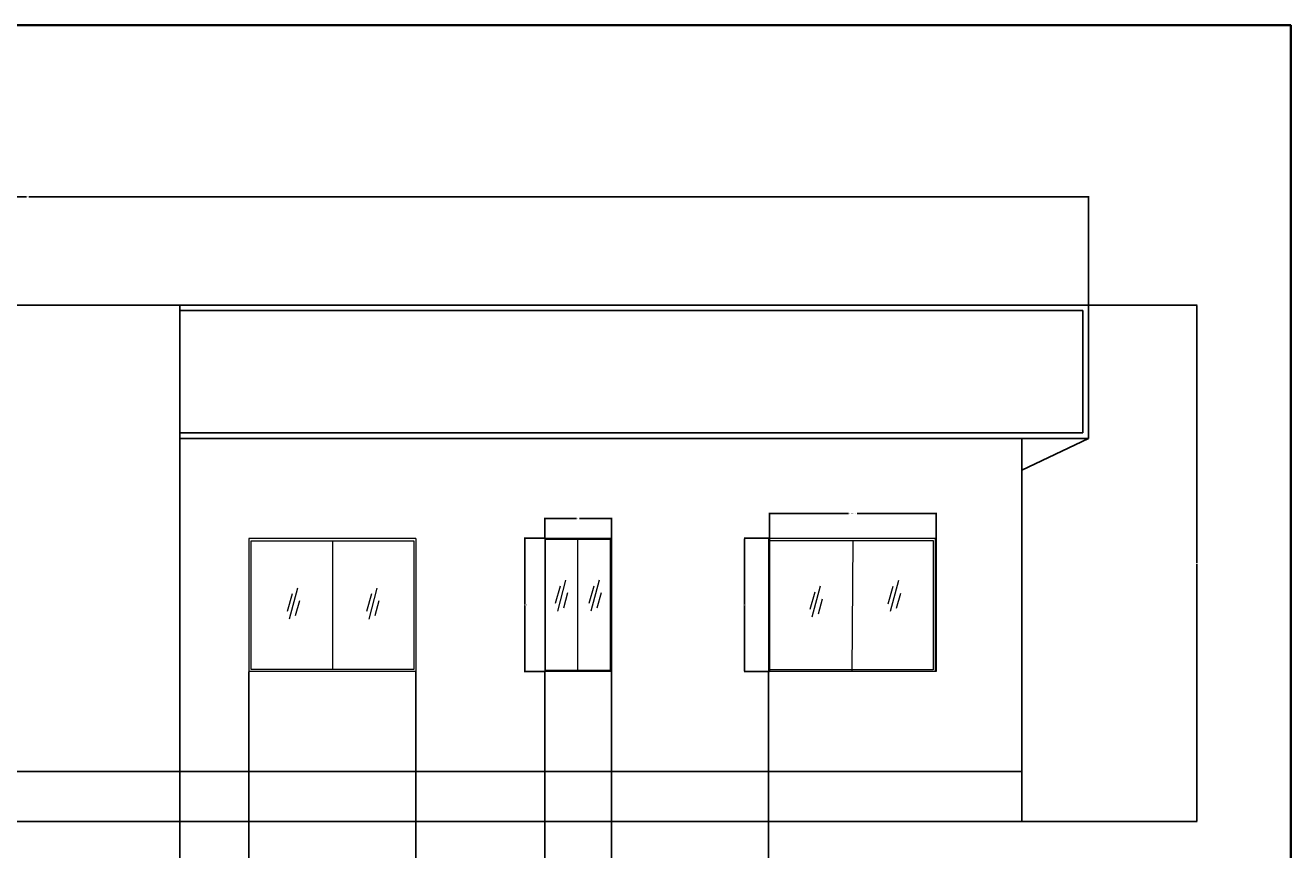
# Model space of a CAD drawing. Units: inches. Extents: x 2314 to 3223, y 1382 to 2735.
# Tile 14 of 14: x 2767 to 3223, y 2439 to 2735. Entities that reach past the tile are written whole.
import ezdxf

# ---------------------------------------------------------------- set-up
doc = ezdxf.new("R2010")
doc.units = ezdxf.units.IN
for name, color, linetype, lineweight in [('A-ANNO-DIMS', 2, 'Continuous', 18), ('A-ANNO-TTLB', 7, 'Continuous', 35), ('A-ELEV', 7, 'Continuous', 25), ('A-GLAZ-ELEV', 4, 'Continuous', 18)]:
    doc.layers.add(name, color=color, linetype=linetype, lineweight=lineweight)
doc.styles.get("Standard").update_dxf_attribs({"font": 'arial.ttf'})
doc.dimstyles.get("Standard").update_dxf_attribs({"dimtxt": 0.18, "dimasz": 0.18, "dimexe": 0.18, "dimexo": 0.0625, "dimgap": 0.09, "dimtad": 0, "dimtih": 1, "dimtoh": 1, "dimdec": 4, "dimzin": 0, "dimdsep": 46, "dimtxsty": 'Standard', "dimcen": 0.09, "dimadec": 0, "dimazin": 0, "dimtfac": 1, "dimtdec": 4, "dimtofl": 0, "dimtmove": 0, "dimatfit": 3, "dimfxl": 1, "dimtolj": 1, "dimtzin": 0, "dimarcsym": 0})

# ---------------------------------------------------------------- blocks, each defined once
blk = doc.blocks.new('WIN-ELEV-60X48-DIVIDED')
for p, q in [((0, 48), (0, 0)), ((60, 48), (0, 48)), ((30.07, 47.13), (30.07, 0.71)), ((60, 48), (60, 0)), ((60, 0), (0, 0))]:
    blk.add_line(p, q)
blk.add_lwpolyline([(0.83, 47.13), (59.31, 47.13), (59.31, 0.71), (0.83, 0.71)], close=True)
blk = doc.blocks.new('WIN-ELEV-60X48-FRAME-SASH')
for p, q in [((0, 48), (0, 0)), ((60, 48), (0, 48)), ((60, 48), (60, 0)), ((60, 0), (0, 0))]:
    blk.add_line(p, q)
blk.add_lwpolyline([(0.54, 47.23), (59.34, 47.23), (59.34, 0.63), (0.54, 0.63)], close=True)
blk = doc.blocks.new('WIN-ELEV-24X48-FRAME')
for p, q in [((0, 48), (0, 0)), ((24, 48), (0, 48)), ((24, 48), (24, 0)), ((24, 0), (0, 0))]:
    blk.add_line(p, q)
blk = doc.blocks.new('WIN-ELEV-60X48-FRAME')
for p, q in [((0, 48), (0, 0)), ((60, 48), (0, 48)), ((60, 48), (60, 0)), ((60, 0), (0, 0))]:
    blk.add_line(p, q)
blk = doc.blocks.new('GLASS-REFLECTION-MARK')
for p, q in [((3.77, 11.17), (0.81, 0)), ((1.83, 9.04), (0, 2.74)), ((4.5, 6.57), (2.99, 1.12))]:
    blk.add_line(p, q)
blk = doc.blocks.new('*D25')
at = {"layer": 'A-ANNO-DIMS', "color": 0, "lineweight": -2, "transparency": 16777216}
for p, q in [((2954.16, 2550.68), (2946.84, 2550.68)), ((2947.02, 2550.5), (2947.02, 2526.86)), ((2947.02, 2502.86), (2947.02, 2526.5)), ((2954.16, 2502.68), (2946.84, 2502.68))]:
    blk.add_line(p, q, dxfattribs=at)
at = {"layer": 'A-ANNO-DIMS', "color": 0, "transparency": 16777216}
for points in [[(2946.99, 2550.5), (2947.05, 2550.5), (2947.02, 2550.68)], [(2946.99, 2502.86), (2947.05, 2502.86), (2947.02, 2502.68)]]:
    blk.add_solid(points, dxfattribs=at)
at = {"layer": 'Defpoints', "color": 0, "transparency": 16777216}
for p in [(2947.02, 2550.68), (2954.22, 2550.68), (2954.22, 2502.68)]:
    blk.add_point(p, dxfattribs=at)
at = {"layer": 'A-ANNO-DIMS', "color": 0, "transparency": 16777216, "insert": (2947.02, 2526.68), "char_height": 0.18, "attachment_point": 5}
blk.add_mtext('\\A1;WINDOW 48 TYP.', dxfattribs=at)
blk = doc.blocks.new('*D26')
at = {"layer": 'A-ANNO-DIMS', "color": 0, "lineweight": -2, "transparency": 16777216}
for p, q in [((2954.22, 2550.74), (2954.22, 2558.06)), ((2954.4, 2557.88), (2965.69, 2557.88)), ((2978.04, 2557.88), (2966.75, 2557.88)), ((2978.22, 2550.74), (2978.22, 2558.06))]:
    blk.add_line(p, q, dxfattribs=at)
at = {"layer": 'A-ANNO-DIMS', "color": 0, "transparency": 16777216}
for points in [[(2954.4, 2557.91), (2954.4, 2557.85), (2954.22, 2557.88)], [(2978.04, 2557.91), (2978.04, 2557.85), (2978.22, 2557.88)]]:
    blk.add_solid(points, dxfattribs=at)
at = {"layer": 'Defpoints', "color": 0, "transparency": 16777216}
for p in [(2978.22, 2557.88), (2954.22, 2550.68), (2978.22, 2550.68)]:
    blk.add_point(p, dxfattribs=at)
at = {"layer": 'A-ANNO-DIMS', "color": 0, "transparency": 16777216, "insert": (2966.22, 2557.88), "char_height": 0.18, "attachment_point": 5}
blk.add_mtext('\\A1;24 TYP.', dxfattribs=at)
blk = doc.blocks.new('*D27')
at = {"layer": 'A-ANNO-DIMS', "color": 0, "lineweight": -2, "transparency": 16777216}
for p, q in [((3035.12, 2550.74), (3035.12, 2559.86)), ((3035.3, 2559.68), (3063.52, 2559.68)), ((3094.94, 2559.68), (3066.71, 2559.68)), ((3095.12, 2550.74), (3095.12, 2559.86))]:
    blk.add_line(p, q, dxfattribs=at)
at = {"layer": 'A-ANNO-DIMS', "color": 0, "transparency": 16777216}
for points in [[(3035.3, 2559.71), (3035.3, 2559.65), (3035.12, 2559.68)], [(3094.94, 2559.71), (3094.94, 2559.65), (3095.12, 2559.68)]]:
    blk.add_solid(points, dxfattribs=at)
at = {"layer": 'Defpoints', "color": 0, "transparency": 16777216}
for p in [(3095.12, 2559.68), (3035.12, 2550.68), (3095.12, 2550.68)]:
    blk.add_point(p, dxfattribs=at)
at = {"layer": 'A-ANNO-DIMS', "color": 0, "transparency": 16777216, "insert": (3065.12, 2559.68), "char_height": 0.18, "attachment_point": 5}
blk.add_mtext('\\A1;WINDOW FRAME 60 TYP.', dxfattribs=at)
blk = doc.blocks.new('*D28')
at = {"layer": 'A-ANNO-DIMS', "color": 0, "lineweight": -2, "transparency": 16777216}
for p, q in [((3035.05, 2550.68), (3025.94, 2550.68)), ((3026.12, 2550.5), (3026.12, 2526.86)), ((3026.12, 2502.86), (3026.12, 2526.5)), ((3035.05, 2502.68), (3025.94, 2502.68))]:
    blk.add_line(p, q, dxfattribs=at)
at = {"layer": 'A-ANNO-DIMS', "color": 0, "transparency": 16777216}
for points in [[(3026.09, 2550.5), (3026.15, 2550.5), (3026.12, 2550.68)], [(3026.09, 2502.86), (3026.15, 2502.86), (3026.12, 2502.68)]]:
    blk.add_solid(points, dxfattribs=at)
at = {"layer": 'Defpoints', "color": 0, "transparency": 16777216}
for p in [(3026.12, 2550.68), (3035.12, 2550.68), (3035.12, 2502.68)]:
    blk.add_point(p, dxfattribs=at)
at = {"layer": 'A-ANNO-DIMS', "color": 0, "transparency": 16777216, "insert": (3026.12, 2526.68), "char_height": 0.18, "attachment_point": 5}
blk.add_mtext('\\A1;48 TYP.', dxfattribs=at)
blk = doc.blocks.new('*D46')
at = {"layer": 'A-ANNO-DIMS', "color": 0, "lineweight": -2, "transparency": 16777216}
for p, q in [((2386.39, 2634.74), (2386.39, 2673.86)), ((2386.57, 2673.68), (2767.75, 2673.68)), ((3149.71, 2673.68), (2768.54, 2673.68)), ((3149.89, 2634.74), (3149.89, 2673.86))]:
    blk.add_line(p, q, dxfattribs=at)
at = {"layer": 'A-ANNO-DIMS', "color": 0, "transparency": 16777216}
for points in [[(2386.57, 2673.71), (2386.57, 2673.65), (2386.39, 2673.68)], [(3149.71, 2673.71), (3149.71, 2673.65), (3149.89, 2673.68)]]:
    blk.add_solid(points, dxfattribs=at)
at = {"layer": 'Defpoints', "color": 0, "transparency": 16777216}
for p in [(3149.89, 2673.68), (2386.39, 2634.68), (3149.89, 2634.68)]:
    blk.add_point(p, dxfattribs=at)
at = {"layer": 'A-ANNO-DIMS', "color": 0, "transparency": 16777216, "insert": (2768.14, 2673.68), "char_height": 0.18, "attachment_point": 5}
blk.add_mtext('\\A1;763.5', dxfattribs=at)
blk = doc.blocks.new('*D47')
at = {"layer": 'A-ANNO-DIMS', "color": 0, "lineweight": -2, "transparency": 16777216}
for p, q in [((3149.96, 2634.68), (3189.07, 2634.68)), ((3188.89, 2634.5), (3188.89, 2541.86)), ((3188.89, 2448.86), (3188.89, 2541.5)), ((3125.96, 2448.68), (3189.07, 2448.68))]:
    blk.add_line(p, q, dxfattribs=at)
at = {"layer": 'A-ANNO-DIMS', "color": 0, "transparency": 16777216}
for points in [[(3188.86, 2634.5), (3188.92, 2634.5), (3188.89, 2634.68)], [(3188.86, 2448.86), (3188.92, 2448.86), (3188.89, 2448.68)]]:
    blk.add_solid(points, dxfattribs=at)
at = {"layer": 'Defpoints', "color": 0, "transparency": 16777216}
for p in [(3149.89, 2634.68), (3125.89, 2448.68), (3188.89, 2448.68)]:
    blk.add_point(p, dxfattribs=at)
at = {"layer": 'A-ANNO-DIMS', "color": 0, "transparency": 16777216, "insert": (3188.89, 2541.68), "char_height": 0.18, "attachment_point": 5}
blk.add_mtext('\\A1;186', dxfattribs=at)
blk = doc.blocks.new('*D56')
at = {"layer": 'A-ANNO-DIMS', "color": 0, "lineweight": -2, "transparency": 16777216}
for p, q in [((2717.89, 2466.62), (2717.89, 2371.63)), ((2822.89, 2466.62), (2822.89, 2371.63)), ((2718.07, 2371.81), (2770.11, 2371.81)), ((2822.71, 2371.81), (2770.67, 2371.81))]:
    blk.add_line(p, q, dxfattribs=at)
at = {"layer": 'A-ANNO-DIMS', "color": 0, "transparency": 16777216}
for points in [[(2718.07, 2371.84), (2718.07, 2371.78), (2717.89, 2371.81)], [(2822.71, 2371.84), (2822.71, 2371.78), (2822.89, 2371.81)]]:
    blk.add_solid(points, dxfattribs=at)
at = {"layer": 'Defpoints', "color": 0, "transparency": 16777216}
for p in [(2717.89, 2466.68), (2822.89, 2466.68), (2822.89, 2371.81)]:
    blk.add_point(p, dxfattribs=at)
at = {"layer": 'A-ANNO-DIMS', "color": 0, "transparency": 16777216, "insert": (2770.39, 2371.81), "char_height": 0.18, "attachment_point": 5}
blk.add_mtext('\\A1;105', dxfattribs=at)
blk = doc.blocks.new('*D57')
at = {"layer": 'A-ANNO-DIMS', "color": 0, "lineweight": -2, "transparency": 16777216}
for p, q in [((2847.78, 2502.62), (2847.78, 2371.63)), ((2822.89, 2466.62), (2822.89, 2371.63)), ((2823.07, 2371.81), (2834.94, 2371.81)), ((2847.6, 2371.81), (2835.73, 2371.81))]:
    blk.add_line(p, q, dxfattribs=at)
at = {"layer": 'A-ANNO-DIMS', "color": 0, "transparency": 16777216}
for points in [[(2823.07, 2371.84), (2823.07, 2371.78), (2822.89, 2371.81)], [(2847.6, 2371.84), (2847.6, 2371.78), (2847.78, 2371.81)]]:
    blk.add_solid(points, dxfattribs=at)
at = {"layer": 'Defpoints', "color": 0, "transparency": 16777216}
for p in [(2847.78, 2502.68), (2822.89, 2466.68), (2847.78, 2371.81)]:
    blk.add_point(p, dxfattribs=at)
at = {"layer": 'A-ANNO-DIMS', "color": 0, "transparency": 16777216, "insert": (2835.34, 2371.81), "char_height": 0.18, "attachment_point": 5}
blk.add_mtext('\\A1;24.89', dxfattribs=at)
blk = doc.blocks.new('*D58')
at = {"layer": 'A-ANNO-DIMS', "color": 0, "lineweight": -2, "transparency": 16777216}
for p, q in [((2907.78, 2502.62), (2907.78, 2371.63)), ((2954.22, 2502.62), (2954.22, 2371.63)), ((2907.96, 2371.81), (2930.61, 2371.81)), ((2954.04, 2371.81), (2931.4, 2371.81))]:
    blk.add_line(p, q, dxfattribs=at)
at = {"layer": 'A-ANNO-DIMS', "color": 0, "transparency": 16777216}
for points in [[(2907.96, 2371.84), (2907.96, 2371.78), (2907.78, 2371.81)], [(2954.04, 2371.84), (2954.04, 2371.78), (2954.22, 2371.81)]]:
    blk.add_solid(points, dxfattribs=at)
at = {"layer": 'Defpoints', "color": 0, "transparency": 16777216}
for p in [(2907.78, 2502.68), (2954.22, 2502.68), (2954.22, 2371.81)]:
    blk.add_point(p, dxfattribs=at)
at = {"layer": 'A-ANNO-DIMS', "color": 0, "transparency": 16777216, "insert": (2931, 2371.81), "char_height": 0.18, "attachment_point": 5}
blk.add_mtext('\\A1;46.44', dxfattribs=at)
blk = doc.blocks.new('*D59')
at = {"layer": 'A-ANNO-DIMS', "color": 0, "lineweight": -2, "transparency": 16777216}
for p, q in [((2978.22, 2502.62), (2978.22, 2371.63)), ((3034.7, 2502.62), (3034.7, 2371.63)), ((2978.4, 2371.81), (3006.07, 2371.81)), ((3034.52, 2371.81), (3006.85, 2371.81))]:
    blk.add_line(p, q, dxfattribs=at)
at = {"layer": 'A-ANNO-DIMS', "color": 0, "transparency": 16777216}
for points in [[(2978.4, 2371.84), (2978.4, 2371.78), (2978.22, 2371.81)], [(3034.52, 2371.84), (3034.52, 2371.78), (3034.7, 2371.81)]]:
    blk.add_solid(points, dxfattribs=at)
at = {"layer": 'Defpoints', "color": 0, "transparency": 16777216}
for p in [(2978.22, 2502.68), (3034.7, 2502.68), (3034.7, 2371.81)]:
    blk.add_point(p, dxfattribs=at)
at = {"layer": 'A-ANNO-DIMS', "color": 0, "transparency": 16777216, "insert": (3006.46, 2371.81), "char_height": 0.18, "attachment_point": 5}
blk.add_mtext('\\A1;56.47', dxfattribs=at)

msp = doc.modelspace()

# ---------------------------------------------------------------- linework, layer by layer
at = {"layer": 'A-ANNO-TTLB'}
msp.add_lwpolyline([(2314.008, 2735.417), (3222.6676, 2735.417), (3222.6676, 1382.0876), (2314.008, 1382.0876)], close=True, dxfattribs=at)
at = {"layer": 'A-ELEV'}
for p, q in [((3149.8927, 2634.6793), (2386.3927, 2634.6793)), ((2822.8927, 2586.6793), (2822.8927, 2634.6793)), ((2822.8927, 2632.6793), (3147.8927, 2632.6793)), ((3147.8927, 2632.6793), (3147.8927, 2588.6793)), ((3149.8927, 2586.6793), (3149.8927, 2634.6793)), ((3147.8927, 2588.6793), (2822.8927, 2588.6793)), ((2822.8927, 2586.6793), (2822.8927, 2466.6793)), ((3149.8927, 2586.6793), (2822.8927, 2586.6793)), ((3125.8927, 2586.6793), (3125.8927, 2448.6793)), ((3149.8927, 2586.6793), (3125.8927, 2575.1733)), ((3125.8927, 2466.6793), (2410.3927, 2466.6793)), ((3125.8927, 2448.6793), (2410.3927, 2448.6793))]:
    msp.add_line(p, q, dxfattribs=at)
at = {"layer": 'A-GLAZ-ELEV'}
for p, q in [((2966.1716, 2503.0629), (2966.1716, 2550.3487)), ((3065.116, 2549.9127), (3064.6958, 2502.6793))]:
    msp.add_line(p, q, dxfattribs=at)
msp.add_lwpolyline([(2954.547, 2550.3487), (2977.7963, 2550.3487), (2977.7963, 2503.0629), (2954.547, 2503.0629)], close=True, dxfattribs=at)

# ---------------------------------------------------------------- block references
for name, p in [('WIN-ELEV-60X48-DIVIDED', (2847.783, 2502.6793)), ('WIN-ELEV-60X48-FRAME', (2847.783, 2502.6793)), ('WIN-ELEV-24X48-FRAME', (2954.2225, 2502.6793)), ('WIN-ELEV-60X48-FRAME-SASH', (3034.6958, 2502.6793)), ('WIN-ELEV-60X48-FRAME', (3035.116, 2502.6793)), ('GLASS-REFLECTION-MARK', (2861.4781, 2521.617)), ('GLASS-REFLECTION-MARK', (2890.075, 2521.617)), ('GLASS-REFLECTION-MARK', (2957.9525, 2524.4674)), ('GLASS-REFLECTION-MARK', (2970.0356, 2524.4674)), ('GLASS-REFLECTION-MARK', (3049.5843, 2522.2635)), ('GLASS-REFLECTION-MARK', (3077.7113, 2524.2771))]:
    msp.add_blockref(name, p, dxfattribs=at)

# ---------------------------------------------------------------- dimensions: what is measured, and where the dimension line sits
at = {"layer": 'A-ANNO-DIMS'}
for base, p1, p2, override, picture, middle in [((3149.8927, 2673.6793), (2386.3927, 2634.6793), (3149.8927, 2634.6793), {"dimdec": 1, "dimlfac": 1, "dimrnd": 0, "dimzin": 0, "dimdsep": 46, "dimlunit": 2}, '*D46', (2768.1427, 2673.6793)), ((2847.783, 2371.8121), (2822.8927, 2466.6793), (2847.783, 2502.6793), {"dimdec": 2, "dimlfac": 1, "dimrnd": 0, "dimzin": 0, "dimdsep": 46, "dimlunit": 2}, '*D57', (2835.3378, 2371.8121)), ((2954.2225, 2371.8121), (2907.783, 2502.6793), (2954.2225, 2502.6793), {"dimdec": 2, "dimlfac": 1, "dimrnd": 0, "dimzin": 0, "dimdsep": 46, "dimlunit": 2}, '*D58', (2931.0028, 2371.8121)), ((3034.6958, 2371.8121), (2978.2225, 2502.6793), (3034.6958, 2502.6793), {"dimdec": 2, "dimlfac": 1, "dimrnd": 0, "dimzin": 0, "dimdsep": 46, "dimlunit": 2}, '*D59', (3006.4592, 2371.8121)), ((2822.8927, 2371.8121), (2717.8927, 2466.6793), (2822.8927, 2466.6793), {"dimdec": 0, "dimlfac": 1, "dimrnd": 0, "dimzin": 0, "dimdsep": 46, "dimlunit": 2}, '*D56', (2770.3927, 2371.8121))]:
    dim = msp.add_linear_dim(base=base, p1=p1, p2=p2, dimstyle='Standard', override=override, dxfattribs=at)
    dim.commit()
    dim.dimension.update_dxf_attribs({"geometry": picture, "text_midpoint": middle})
dim = msp.add_linear_dim(base=(3188.8927, 2448.6793), p1=(3149.8927, 2634.6793), p2=(3125.8927, 2448.6793), angle=90, dimstyle='Standard', override={"dimdec": 0, "dimlfac": 1, "dimrnd": 0, "dimzin": 0, "dimdsep": 46, "dimlunit": 2}, dxfattribs=at)
dim.commit()
dim.dimension.update_dxf_attribs({"geometry": '*D47', "text_midpoint": (3188.8927, 2541.6793)})
for base, p1, p2, text, picture, middle in [((3095.116, 2559.6793), (3035.116, 2550.6793), (3095.116, 2550.6793), 'WINDOW FRAME <> TYP.', '*D27', (3065.116, 2559.6793)), ((2978.2225, 2557.8793), (2954.2225, 2550.6793), (2978.2225, 2550.6793), '<> TYP.', '*D26', (2966.2225, 2557.8793))]:
    dim = msp.add_linear_dim(base=base, p1=p1, p2=p2, text=text, dimstyle='Standard', override={"dimdec": 0, "dimlfac": 1, "dimrnd": 0, "dimzin": 0, "dimdsep": 46, "dimlunit": 2}, dxfattribs=at)
    dim.commit()
    dim.dimension.update_dxf_attribs({"geometry": picture, "text_midpoint": middle})
for base, p1, p2, text, picture, middle in [((2947.0225, 2550.6793), (2954.2225, 2502.6793), (2954.2225, 2550.6793), 'WINDOW <> TYP.', '*D25', (2947.0225, 2526.6793)), ((3026.116, 2550.6793), (3035.116, 2502.6793), (3035.116, 2550.6793), '<> TYP.', '*D28', (3026.116, 2526.6793))]:
    dim = msp.add_linear_dim(base=base, p1=p1, p2=p2, angle=90, text=text, dimstyle='Standard', override={"dimdec": 0, "dimlfac": 1, "dimrnd": 0, "dimzin": 0, "dimdsep": 46, "dimlunit": 2}, dxfattribs=at)
    dim.commit()
    dim.dimension.update_dxf_attribs({"geometry": picture, "text_midpoint": middle})

doc.saveas('drawing.dxf')
